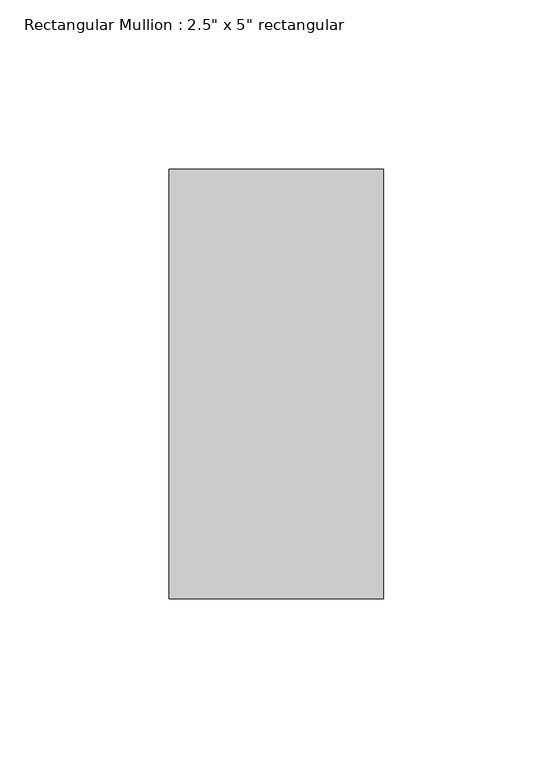
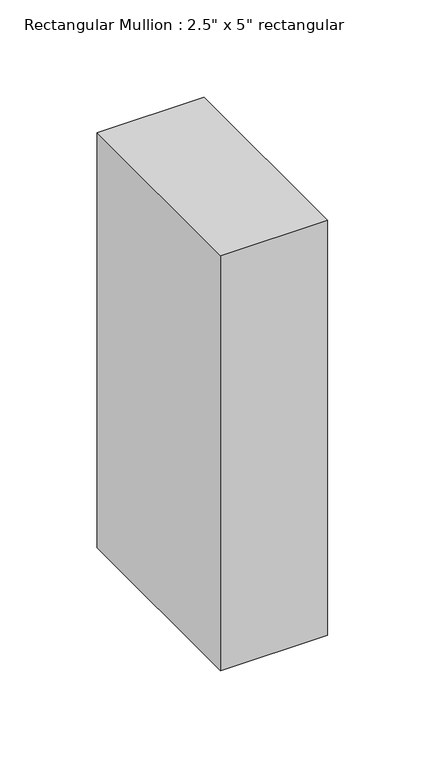
"""IFC4 building model written with IfcOpenShell, lengths in millimetres: member geometry."""

from ifc_helpers import new_model, si_unit, frame, origin, place, context, project, spatial, polyline, outline, extrude, source, transform, mapped, element, save


def member_be2dbdeb(model_context):
    return source(origin(), model_context, "Body", "SweptSolid", [
        extrude(outline(polyline([(31.75, 63.5), (31.75, -63.5), (-31.75, -63.5), (-31.75, 63.5), (31.75, 63.5)])), frame((0.0, 0.0, -260.35), z_axis=(0.0, 0.0, 1.0), x_axis=(1.0, 0.0, 0.0)), (0.0, 0.0, 1.0), 260.35),
    ])


if __name__ == "__main__":
    model = new_model("IFC4")
    model_context = context("Model", 3, world=origin())
    ifc_project = project(units=[si_unit("LENGTHUNIT", "METRE", prefix="MILLI")], contexts=[model_context])
    site = spatial("IfcSite", under=ifc_project)
    building = spatial("IfcBuilding", under=site)
    placement = place(None, origin())
    member_shape = member_be2dbdeb(model_context)
    element("IfcMember", 1, ObjectType="Rectangular Mullion : 2.5\" x 5\" rectangular", at=placement, inside=building, context=model_context, shape_type="MappedRepresentation", body=[
        mapped(member_shape, transform((0.0, 0.0, 0.0), x_axis=(1.0, 0.0, 0.0), y_axis=(0.0, 1.0, 0.0), z_axis=(0.0, 0.0, 1.0))),
    ])
    save(model, "model.ifc")

# Revit data of these elements
# Type "Rectangular Mullion : 2.5\" x 5\" rectangular"
#   built-in parameter 1007304 = 0.416667 (stored number, unit not read)
#   built-in parameter 1007301 = 0.104167 (stored number, unit not read)
#   built-in parameter 1007300 = 0.104167 (stored number, unit not read)
